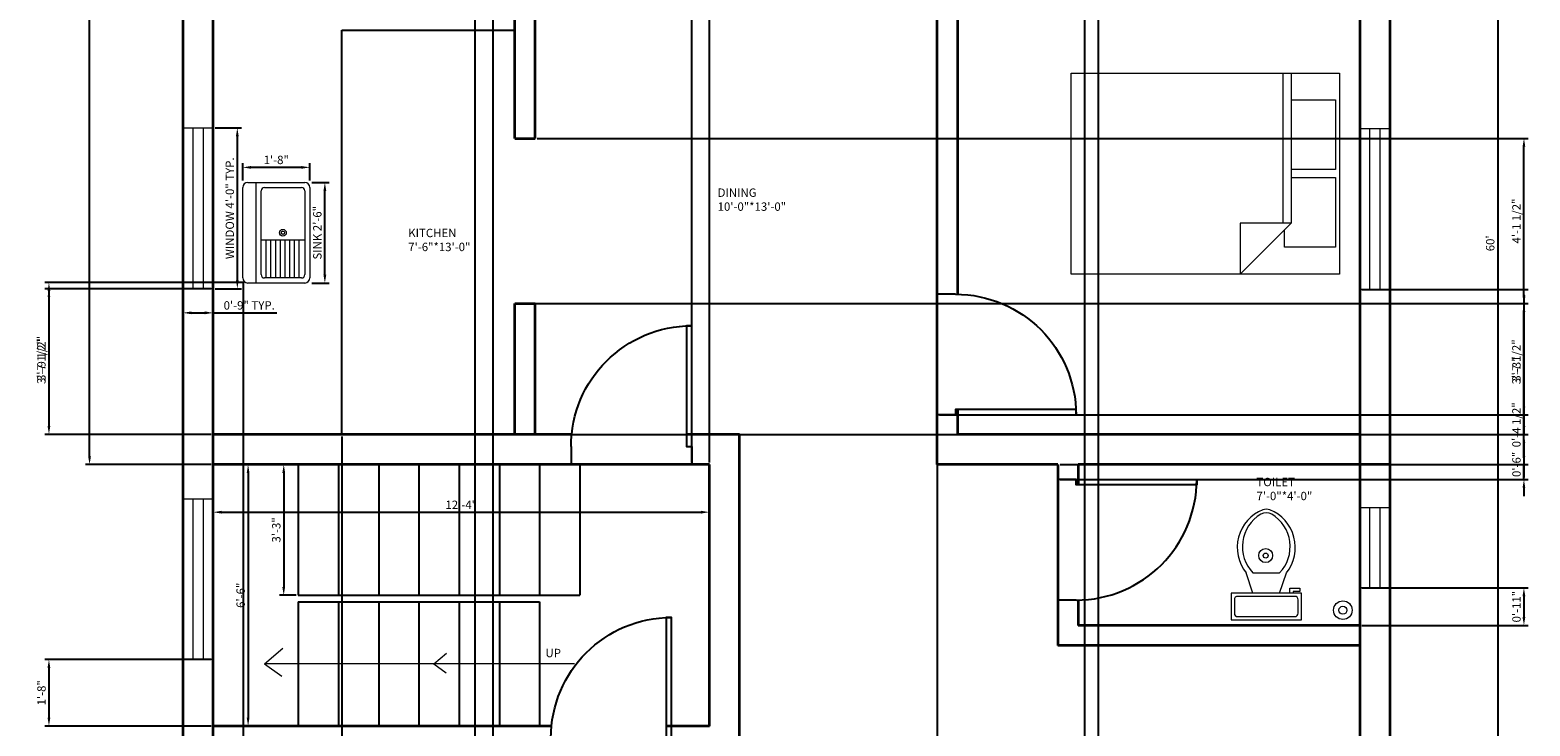
# Model space of a CAD drawing. Units: inches. Extents: x 2162 to 2610, y 1546 to 2356.
# Tile 2 of 3: x 2162 to 2610, y 1804 to 2012. Entities that reach past the tile are written whole.
import ezdxf

# ---------------------------------------------------------------- set-up
doc = ezdxf.new("R2010")
doc.units = ezdxf.units.IN
for name, color, linetype, lineweight in [('A-ANNO-DIMS', 2, 'Continuous', 18), ('A-ANNO-SYMB', 7, 'Continuous', 18), ('A-ANNO-TEXT', 7, 'Continuous', 25), ('A-AREA-IDEN', 7, 'Continuous', 18), ('A-DOOR', 3, 'Continuous', 25), ('A-FLOR-CASE', 8, 'Continuous', 25), ('A-FLOR-FIXT', 9, 'Continuous', 18), ('A-FLOR-STRS', 7, 'Continuous', 25), ('A-FURN', 8, 'Continuous', 18), ('A-GLAZ', 4, 'Continuous', 18), ('A-WALL', 7, 'Continuous', 35)]:
    doc.layers.add(name, color=color, linetype=linetype, lineweight=lineweight)
doc.styles.get("Standard").update_dxf_attribs({"font": 'arial.ttf'})
doc.dimstyles.new('ISO-25', dxfattribs={"dimtxt": 2.5, "dimasz": 2.5, "dimexe": 1.25, "dimexo": 0.625, "dimtad": 1, "dimdec": 1, "dimlunit": 3, "dimtxsty": 'Standard', "dimcen": 2.5, "dimadec": 0, "dimazin": 0, "dimtfac": 1, "dimtdec": 1, "dimtmove": 0, "dimatfit": 3, "dimfxl": 1, "dimarcsym": 0})

# ---------------------------------------------------------------- blocks, each defined once
blk = doc.blocks.new('*U2')
for p, q in [((0, 0), (0, -6)), ((40, 0), (40, -6))]:
    blk.add_line(p, q)
blk.add_lwpolyline([(0, 0), (0, 40), (1.75, 40), (1.75, 0)], close=True)
blk.add_arc((0, 0), 40, 0, 90)
blk = doc.blocks.new('*D4')
at = {"layer": 'A-ANNO-DIMS', "color": 0, "lineweight": -2, "transparency": 16777216}
for p, q in [((2216.24, 2308.05), (2178.74, 2308.05)), ((2179.99, 1884.55), (2179.99, 2305.55)), ((2216.24, 1882.05), (2178.74, 1882.05))]:
    blk.add_line(p, q, dxfattribs=at)
at = {"layer": 'A-ANNO-DIMS', "color": 0, "transparency": 16777216}
for points in [[(2179.57, 2305.55), (2180.4, 2305.55), (2179.99, 2308.05)], [(2179.57, 1884.55), (2180.4, 1884.55), (2179.99, 1882.05)]]:
    blk.add_solid(points, dxfattribs=at)
at = {"layer": 'Defpoints', "color": 0, "transparency": 16777216}
for p in [(2179.99, 2308.05), (2216.87, 2308.05), (2216.87, 1882.05)]:
    blk.add_point(p, dxfattribs=at)
at = {"layer": 'A-ANNO-DIMS', "color": 0, "transparency": 16777216, "insert": (2178.09, 2095.05), "char_height": 2.5, "attachment_point": 5, "rotation": 90}
blk.add_mtext('35\'-6"', dxfattribs=at)
blk = doc.blocks.new('*D5')
at = {"layer": 'A-ANNO-DIMS', "color": 0, "lineweight": -2, "transparency": 16777216}
for p, q in [((2568.49, 2308.05), (2601.29, 2308.05)), ((2600.04, 2305.55), (2600.04, 1590.55)), ((2568.49, 1588.05), (2601.29, 1588.05))]:
    blk.add_line(p, q, dxfattribs=at)
at = {"layer": 'A-ANNO-DIMS', "color": 0, "transparency": 16777216}
for points in [[(2599.62, 2305.55), (2600.45, 2305.55), (2600.04, 2308.05)], [(2599.62, 1590.55), (2600.45, 1590.55), (2600.04, 1588.05)]]:
    blk.add_solid(points, dxfattribs=at)
at = {"layer": 'Defpoints', "color": 0, "transparency": 16777216}
for p in [(2567.87, 2308.05), (2567.87, 1588.05), (2600.04, 1588.05)]:
    blk.add_point(p, dxfattribs=at)
at = {"layer": 'A-ANNO-DIMS', "color": 0, "transparency": 16777216, "insert": (2598.14, 1948.05), "char_height": 2.5, "attachment_point": 5, "rotation": 90}
blk.add_mtext("60'", dxfattribs=at)
blk = doc.blocks.new('Bed - Queen')
for p, q in [((0, -80.00003), (0, 0)), ((0, 0), (59.99999, 0)), ((59.99999, 0), (59.99999, -80.00003)), ((7.99999, -1.2), (28.79998, -1.2)), ((7.99999, -14.4), (7.99999, -1.2)), ((28.79998, -1.2), (28.79998, -14.4)), ((31.19999, -1.2), (51.99999, -1.2)), ((31.19999, -14.4), (31.19999, -1.2)), ((51.99999, -1.2), (51.99999, -16.4)), ((0, -14.4), (44.8, -14.4)), ((44.8, -16.8), (0, -16.8)), ((59.99999, -29.6), (44.8, -14.4)), ((44.8, -14.4), (44.8, -29.6)), ((51.99999, -16.4), (46.79936, -16.4)), ((44.8, -29.6), (59.99999, -29.6)), ((59.99999, -80.00003), (0, -80.00003))]:
    blk.add_line(p, q)
blk = doc.blocks.new('Toilet - top')
for p, q in [((9.5, -6), (9.5, -2)), ((-10, -8.5), (-8, -8.5)), ((-10, -9.5), (-10, -8.5)), ((-8, -8.5), (-8, -8)), ((-7, -8), (-7, -9.5)), ((-4, -8), (-6, -14)), ((4, -8), (6, -14)), ((-7, -9.5), (-10, -9.5)), ((4, -14), (-4, -14))]:
    blk.add_line(p, q)
blk.add_lwpolyline([(10.5, -8), (10.5, 0), (-10.5, 0), (-10.5, -8)], close=True)
for points in [[(-9.5, -2), (-9.5, -6)], [(8.5, -1), (-8.5, -1)], [(-8.5, -7), (8.5, -7)]]:
    blk.add_lwpolyline(points)
for centre, radius, start, end in [((-8.62, -1.88), 0.884, 81.8699, 188.1301), ((8.62, -1.88), 0.884, 351.8699, 98.1301), ((-8.62, -6.12), 0.884, 171.8699, 278.1301), ((8.62, -6.12), 0.884, 261.8699, 8.1301), ((3.52, -21.58), 12.17, 141.4691, 247.9714), ((4.2, -21.82), 11.33, 136.3677, 238.9468), ((-3.52, -21.58), 12.17, 292.0284, 38.5307), ((-4.2, -21.82), 11.33, 301.053, 43.6321), ((0, -27.88), 4, 245.7318, 294.2682), ((0, -29), 4, 254.8605, 285.1395)]:
    blk.add_arc(centre, radius, start, end)
blk = doc.blocks.new('Sink-single - 30 in top')
blk.add_line((-15, -3.999996), (15, -3.999996))
for points in [[(-13.5, 0), (13.5, 0)], [(-15, -18.499996), (-15, -1.5)], [(15, -1.5), (15, -18.499996)], [(-13.5, -17.499996), (-13.5, -6.499996)], [(-12.5, -5.499996), (12.5, -5.499996)], [(13.5, -6.499996), (13.5, -17.499996)], [(13.5, -19.999996), (-13.5, -19.999996)], [(12.5, -18.499996), (-12.5, -18.499996)]]:
    blk.add_lwpolyline(points)
for radius in [1, 0.5]:
    blk.add_circle((0, -11.999996), radius)
for centre, radius, start, end in [((-13.5, -1.5), 1.5, 90, 180), ((13.5, -1.5), 1.5, 0, 90), ((-12.5, -6.499996), 1, 90, 180), ((12.5, -6.499996), 1, 0, 90), ((-12.5, -17.499996), 1, 180, 270), ((12.5, -17.499996), 1, 270, 0), ((-13.5, -18.499996), 1.5, 180, 270), ((13.5, -18.499996), 1.5, 270, 0)]:
    blk.add_arc(centre, radius, start, end)
blk = doc.blocks.new('*D9')
at = {"layer": 'A-ANNO-DIMS', "color": 0, "lineweight": -2, "transparency": 16777216}
for p, q in [((2226.7, 1882.05), (2228.53, 1882.05)), ((2227.28, 1879.55), (2227.28, 1806.55)), ((2226.7, 1804.05), (2228.53, 1804.05))]:
    blk.add_line(p, q, dxfattribs=at)
at = {"layer": 'A-ANNO-DIMS', "color": 0, "transparency": 16777216}
for points in [[(2226.87, 1879.55), (2227.7, 1879.55), (2227.28, 1882.05)], [(2226.87, 1806.55), (2227.7, 1806.55), (2227.28, 1804.05)]]:
    blk.add_solid(points, dxfattribs=at)
at = {"layer": 'Defpoints', "color": 0, "transparency": 16777216}
for p in [(2226.07, 1882.05), (2226.07, 1804.05), (2227.28, 1804.05)]:
    blk.add_point(p, dxfattribs=at)
at = {"layer": 'A-ANNO-DIMS', "color": 0, "transparency": 16777216, "insert": (2225.38, 1843.05), "char_height": 2.5, "attachment_point": 5, "rotation": 90}
blk.add_mtext('6\'-6"', dxfattribs=at)
blk = doc.blocks.new('*D10')
at = {"layer": 'A-ANNO-DIMS', "color": 0, "lineweight": -2, "transparency": 16777216}
for p, q in [((2241.6, 1882.05), (2236.66, 1882.05)), ((2237.91, 1879.55), (2237.91, 1845.55)), ((2241.6, 1843.05), (2236.66, 1843.05))]:
    blk.add_line(p, q, dxfattribs=at)
at = {"layer": 'A-ANNO-DIMS', "color": 0, "transparency": 16777216}
for points in [[(2237.49, 1879.55), (2238.33, 1879.55), (2237.91, 1882.05)], [(2237.49, 1845.55), (2238.33, 1845.55), (2237.91, 1843.05)]]:
    blk.add_solid(points, dxfattribs=at)
at = {"layer": 'Defpoints', "color": 0, "transparency": 16777216}
for p in [(2242.23, 1882.05), (2237.91, 1843.05), (2242.23, 1843.05)]:
    blk.add_point(p, dxfattribs=at)
at = {"layer": 'A-ANNO-DIMS', "color": 0, "transparency": 16777216, "insert": (2236.01, 1862.55), "char_height": 2.5, "attachment_point": 5, "rotation": 90}
blk.add_mtext('3\'-3"', dxfattribs=at)
blk = doc.blocks.new('*D11')
at = {"layer": 'A-ANNO-DIMS', "color": 0, "lineweight": -2, "transparency": 16777216}
for p, q in [((2216.87, 1881.43), (2216.87, 1866.59)), ((2364.87, 1881.43), (2364.87, 1866.59)), ((2219.37, 1867.84), (2362.37, 1867.84))]:
    blk.add_line(p, q, dxfattribs=at)
at = {"layer": 'A-ANNO-DIMS', "color": 0, "transparency": 16777216}
for points in [[(2219.37, 1868.26), (2219.37, 1867.42), (2216.87, 1867.84)], [(2362.37, 1868.26), (2362.37, 1867.42), (2364.87, 1867.84)]]:
    blk.add_solid(points, dxfattribs=at)
at = {"layer": 'Defpoints', "color": 0, "transparency": 16777216}
for p in [(2216.87, 1882.05), (2364.87, 1882.05), (2364.87, 1867.84)]:
    blk.add_point(p, dxfattribs=at)
at = {"layer": 'A-ANNO-DIMS', "color": 0, "transparency": 16777216, "insert": (2290.87, 1869.72), "char_height": 2.5, "attachment_point": 5}
blk.add_mtext('12\'-4"', dxfattribs=at)
blk = doc.blocks.new('WIN-48IN')
for p, q in [((0, 0), (0, 48)), ((0, 48), (9, 48)), ((3, 0), (3, 48)), ((6, 48), (6, 0)), ((9, 48), (9, 0)), ((9, 0), (0, 0))]:
    blk.add_line(p, q)
blk = doc.blocks.new('WIN-24IN')
for p, q in [((0, 9), (24, 9)), ((0, 0), (0, 9)), ((24, 9), (24, 0)), ((0, 6), (24, 6)), ((24, 3), (0, 3)), ((24, 0), (0, 0))]:
    blk.add_line(p, q)
blk = doc.blocks.new('*D14')
at = {"layer": 'A-ANNO-DIMS', "color": 0, "lineweight": -2, "transparency": 16777216}
for p, q in [((2217.49, 1982.51), (2225.32, 1982.51)), ((2224.07, 1937.01), (2224.07, 1980.01)), ((2217.49, 1934.51), (2225.32, 1934.51))]:
    blk.add_line(p, q, dxfattribs=at)
at = {"layer": 'A-ANNO-DIMS', "color": 0, "transparency": 16777216}
for points in [[(2223.65, 1980.01), (2224.48, 1980.01), (2224.07, 1982.51)], [(2223.65, 1937.01), (2224.48, 1937.01), (2224.07, 1934.51)]]:
    blk.add_solid(points, dxfattribs=at)
at = {"layer": 'Defpoints', "color": 0, "transparency": 16777216}
for p in [(2216.87, 1982.51), (2224.07, 1982.51), (2216.87, 1934.51)]:
    blk.add_point(p, dxfattribs=at)
at = {"layer": 'A-ANNO-DIMS', "color": 0, "transparency": 16777216, "insert": (2222.15, 1958.51), "char_height": 2.5, "attachment_point": 5, "rotation": 90}
blk.add_mtext('WINDOW 4\'-0" TYP.', dxfattribs=at)
blk = doc.blocks.new('*D15')
at = {"layer": 'A-ANNO-DIMS', "color": 0, "lineweight": -2, "transparency": 16777216}
for p, q in [((2207.87, 1933.89), (2207.87, 1926.06)), ((2216.87, 1933.89), (2216.87, 1926.06)), ((2210.37, 1927.31), (2214.37, 1927.31)), ((2216.87, 1927.31), (2235.86, 1927.31))]:
    blk.add_line(p, q, dxfattribs=at)
at = {"layer": 'A-ANNO-DIMS', "color": 0, "transparency": 16777216}
for points in [[(2210.37, 1927.73), (2210.37, 1926.89), (2207.87, 1927.31)], [(2214.37, 1927.73), (2214.37, 1926.89), (2216.87, 1927.31)]]:
    blk.add_solid(points, dxfattribs=at)
at = {"layer": 'Defpoints', "color": 0, "transparency": 16777216}
for p in [(2207.87, 1934.51), (2216.87, 1934.51), (2216.87, 1927.31)]:
    blk.add_point(p, dxfattribs=at)
at = {"layer": 'A-ANNO-DIMS', "color": 0, "transparency": 16777216, "insert": (2227.61, 1929.21), "char_height": 2.5, "attachment_point": 5}
blk.add_mtext('0\'-9" TYP.', dxfattribs=at)
blk = doc.blocks.new('*D22')
at = {"layer": 'A-ANNO-DIMS', "color": 0, "lineweight": -2, "transparency": 16777216}
for p, q in [((2246.3, 1966.21), (2251.43, 1966.21)), ((2250.18, 1938.71), (2250.18, 1963.71)), ((2246.3, 1936.21), (2251.43, 1936.21))]:
    blk.add_line(p, q, dxfattribs=at)
at = {"layer": 'A-ANNO-DIMS', "color": 0, "transparency": 16777216}
for points in [[(2249.76, 1963.71), (2250.6, 1963.71), (2250.18, 1966.21)], [(2249.76, 1938.71), (2250.6, 1938.71), (2250.18, 1936.21)]]:
    blk.add_solid(points, dxfattribs=at)
at = {"layer": 'Defpoints', "color": 0, "transparency": 16777216}
for p in [(2245.68, 1966.21), (2250.18, 1966.21), (2245.68, 1936.21)]:
    blk.add_point(p, dxfattribs=at)
at = {"layer": 'A-ANNO-DIMS', "color": 0, "transparency": 16777216, "insert": (2248.26, 1951.21), "char_height": 2.5, "attachment_point": 5, "rotation": 90}
blk.add_mtext('SINK 2\'-6"', dxfattribs=at)
blk = doc.blocks.new('*D23')
at = {"layer": 'A-ANNO-DIMS', "color": 0, "lineweight": -2, "transparency": 16777216}
for p, q in [((2225.68, 1966.83), (2225.68, 1971.96)), ((2243.18, 1970.71), (2228.18, 1970.71)), ((2245.68, 1966.83), (2245.68, 1971.96))]:
    blk.add_line(p, q, dxfattribs=at)
at = {"layer": 'A-ANNO-DIMS', "color": 0, "transparency": 16777216}
for points in [[(2228.18, 1971.12), (2228.18, 1970.29), (2225.68, 1970.71)], [(2243.18, 1971.12), (2243.18, 1970.29), (2245.68, 1970.71)]]:
    blk.add_solid(points, dxfattribs=at)
at = {"layer": 'Defpoints', "color": 0, "transparency": 16777216}
for p in [(2225.68, 1970.71), (2225.68, 1966.21), (2245.68, 1966.21)]:
    blk.add_point(p, dxfattribs=at)
at = {"layer": 'A-ANNO-DIMS', "color": 0, "transparency": 16777216, "insert": (2235.68, 1972.61), "char_height": 2.5, "attachment_point": 5}
blk.add_mtext('1\'-8"', dxfattribs=at)
blk = doc.blocks.new('*D25')
at = {"layer": 'A-ANNO-DIMS', "color": 0, "lineweight": -2, "transparency": 16777216}
for p, q in [((2313.49, 1979.36), (2609.12, 1979.36)), ((2607.87, 1932.55), (2607.87, 1976.86)), ((2313.49, 1930.05), (2609.12, 1930.05))]:
    blk.add_line(p, q, dxfattribs=at)
at = {"layer": 'A-ANNO-DIMS', "color": 0, "transparency": 16777216}
for points in [[(2607.45, 1976.86), (2608.28, 1976.86), (2607.87, 1979.36)], [(2607.45, 1932.55), (2608.28, 1932.55), (2607.87, 1930.05)]]:
    blk.add_solid(points, dxfattribs=at)
at = {"layer": 'Defpoints', "color": 0, "transparency": 16777216}
for p in [(2312.87, 1979.36), (2607.87, 1979.36), (2312.87, 1930.05)]:
    blk.add_point(p, dxfattribs=at)
at = {"layer": 'A-ANNO-DIMS', "color": 0, "transparency": 16777216, "insert": (2605.95, 1954.71), "char_height": 2.5, "attachment_point": 5, "rotation": 90}
blk.add_mtext('4\'-1 1/2"', dxfattribs=at)
blk = doc.blocks.new('*D26')
at = {"layer": 'A-ANNO-DIMS', "color": 0, "lineweight": -2, "transparency": 16777216}
for p, q in [((2432.87, 1896.22), (2432.87, 1546.8)), ((2373.87, 1890.43), (2373.87, 1546.8)), ((2376.37, 1548.05), (2430.37, 1548.05))]:
    blk.add_line(p, q, dxfattribs=at)
at = {"layer": 'A-ANNO-DIMS', "color": 0, "transparency": 16777216}
for points in [[(2376.37, 1548.47), (2376.37, 1547.63), (2373.87, 1548.05)], [(2430.37, 1548.47), (2430.37, 1547.63), (2432.87, 1548.05)]]:
    blk.add_solid(points, dxfattribs=at)
at = {"layer": 'Defpoints', "color": 0, "transparency": 16777216}
for p in [(2432.87, 1896.85), (2373.87, 1891.05), (2432.87, 1548.05)]:
    blk.add_point(p, dxfattribs=at)
at = {"layer": 'A-ANNO-DIMS', "color": 0, "transparency": 16777216, "insert": (2403.37, 1549.93), "char_height": 2.5, "attachment_point": 5}
blk.add_mtext('4\'-11"', dxfattribs=at)
blk = doc.blocks.new('*D28')
at = {"layer": 'A-ANNO-DIMS', "color": 0, "lineweight": -2, "transparency": 16777216}
for p, q in [((2216.24, 1934.51), (2166.62, 1934.51)), ((2167.87, 1932.01), (2167.87, 1893.55)), ((2216.24, 1891.05), (2166.62, 1891.05))]:
    blk.add_line(p, q, dxfattribs=at)
at = {"layer": 'A-ANNO-DIMS', "color": 0, "transparency": 16777216}
for points in [[(2167.45, 1932.01), (2168.28, 1932.01), (2167.87, 1934.51)], [(2167.45, 1893.55), (2168.28, 1893.55), (2167.87, 1891.05)]]:
    blk.add_solid(points, dxfattribs=at)
at = {"layer": 'Defpoints', "color": 0, "transparency": 16777216}
for p in [(2216.87, 1934.51), (2167.87, 1891.05), (2216.87, 1891.05)]:
    blk.add_point(p, dxfattribs=at)
at = {"layer": 'A-ANNO-DIMS', "color": 0, "transparency": 16777216, "insert": (2165.95, 1912.78), "char_height": 2.5, "attachment_point": 5, "rotation": 90}
blk.add_mtext('3\'-7 1/2"', dxfattribs=at)
blk = doc.blocks.new('*D29')
at = {"layer": 'A-ANNO-DIMS', "color": 0, "lineweight": -2, "transparency": 16777216}
for p, q in [((2216.24, 1823.87), (2166.62, 1823.87)), ((2167.87, 1821.37), (2167.87, 1806.55)), ((2216.24, 1804.05), (2166.62, 1804.05))]:
    blk.add_line(p, q, dxfattribs=at)
at = {"layer": 'A-ANNO-DIMS', "color": 0, "transparency": 16777216}
for points in [[(2167.45, 1821.37), (2168.28, 1821.37), (2167.87, 1823.87)], [(2167.45, 1806.55), (2168.28, 1806.55), (2167.87, 1804.05)]]:
    blk.add_solid(points, dxfattribs=at)
at = {"layer": 'Defpoints', "color": 0, "transparency": 16777216}
for p in [(2216.87, 1823.87), (2167.87, 1804.05), (2216.87, 1804.05)]:
    blk.add_point(p, dxfattribs=at)
at = {"layer": 'A-ANNO-DIMS', "color": 0, "transparency": 16777216, "insert": (2165.97, 1813.96), "char_height": 2.5, "attachment_point": 5, "rotation": 90}
blk.add_mtext('1\'-8"', dxfattribs=at)
blk = doc.blocks.new('*D31')
at = {"layer": 'A-ANNO-DIMS', "color": 0, "lineweight": -2, "transparency": 16777216}
for p, q in [((2559.49, 1934.32), (2609.12, 1934.32)), ((2607.87, 1931.82), (2607.87, 1893.55)), ((2559.49, 1891.05), (2609.12, 1891.05))]:
    blk.add_line(p, q, dxfattribs=at)
at = {"layer": 'A-ANNO-DIMS', "color": 0, "transparency": 16777216}
for points in [[(2607.45, 1931.82), (2608.28, 1931.82), (2607.87, 1934.32)], [(2607.45, 1893.55), (2608.28, 1893.55), (2607.87, 1891.05)]]:
    blk.add_solid(points, dxfattribs=at)
at = {"layer": 'Defpoints', "color": 0, "transparency": 16777216}
for p in [(2558.87, 1934.32), (2558.87, 1891.05), (2607.87, 1891.05)]:
    blk.add_point(p, dxfattribs=at)
at = {"layer": 'A-ANNO-DIMS', "color": 0, "transparency": 16777216, "insert": (2605.95, 1912.69), "char_height": 2.5, "attachment_point": 5, "rotation": 90}
blk.add_mtext('3\'-7 1/2"', dxfattribs=at)
blk = doc.blocks.new('*D32')
at = {"layer": 'A-ANNO-DIMS', "color": 0, "lineweight": -2, "transparency": 16777216}
for p, q in [((2559.49, 1845.27), (2609.12, 1845.27)), ((2607.87, 1842.77), (2607.87, 1836.55)), ((2559.49, 1834.05), (2609.12, 1834.05))]:
    blk.add_line(p, q, dxfattribs=at)
at = {"layer": 'A-ANNO-DIMS', "color": 0, "transparency": 16777216}
for points in [[(2607.45, 1842.77), (2608.28, 1842.77), (2607.87, 1845.27)], [(2607.45, 1836.55), (2608.28, 1836.55), (2607.87, 1834.05)]]:
    blk.add_solid(points, dxfattribs=at)
at = {"layer": 'Defpoints', "color": 0, "transparency": 16777216}
for p in [(2558.87, 1845.27), (2558.87, 1834.05), (2607.87, 1834.05)]:
    blk.add_point(p, dxfattribs=at)
at = {"layer": 'A-ANNO-DIMS', "color": 0, "transparency": 16777216, "insert": (2605.97, 1839.66), "char_height": 2.5, "attachment_point": 5, "rotation": 90}
blk.add_mtext('0\'-11"', dxfattribs=at)
blk = doc.blocks.new('*D40')
at = {"layer": 'A-ANNO-DIMS', "color": 0, "lineweight": -2, "transparency": 16777216}
for p, q in [((2216.87, 1890.43), (2216.87, 1546.8)), ((2255.27, 1890.43), (2255.27, 1546.8)), ((2219.37, 1548.05), (2252.77, 1548.05))]:
    blk.add_line(p, q, dxfattribs=at)
at = {"layer": 'A-ANNO-DIMS', "color": 0, "transparency": 16777216}
for points in [[(2219.37, 1548.47), (2219.37, 1547.63), (2216.87, 1548.05)], [(2252.77, 1548.47), (2252.77, 1547.63), (2255.27, 1548.05)]]:
    blk.add_solid(points, dxfattribs=at)
at = {"layer": 'Defpoints', "color": 0, "transparency": 16777216}
for p in [(2216.87, 1891.05), (2255.27, 1891.05), (2255.27, 1548.05)]:
    blk.add_point(p, dxfattribs=at)
at = {"layer": 'A-ANNO-DIMS', "color": 0, "transparency": 16777216, "insert": (2236.07, 1549.97), "char_height": 2.5, "attachment_point": 5}
blk.add_mtext('3\'-2 1/2"', dxfattribs=at)
blk = doc.blocks.new('*D44')
at = {"layer": 'A-ANNO-DIMS', "color": 0, "lineweight": -2, "transparency": 16777216}
for p, q in [((2307.49, 1930.05), (2609.12, 1930.05)), ((2607.87, 1893.55), (2607.87, 1927.55)), ((2307.49, 1891.05), (2609.12, 1891.05))]:
    blk.add_line(p, q, dxfattribs=at)
at = {"layer": 'A-ANNO-DIMS', "color": 0, "transparency": 16777216}
for points in [[(2607.45, 1927.55), (2608.28, 1927.55), (2607.87, 1930.05)], [(2607.45, 1893.55), (2608.28, 1893.55), (2607.87, 1891.05)]]:
    blk.add_solid(points, dxfattribs=at)
at = {"layer": 'Defpoints', "color": 0, "transparency": 16777216}
for p in [(2306.87, 1930.05), (2607.87, 1930.05), (2306.87, 1891.05)]:
    blk.add_point(p, dxfattribs=at)
at = {"layer": 'A-ANNO-DIMS', "color": 0, "transparency": 16777216, "insert": (2605.96, 1910.55), "char_height": 2.5, "attachment_point": 5, "rotation": 90}
blk.add_mtext('3\'-3"', dxfattribs=at)
blk = doc.blocks.new('*D47')
at = {"layer": 'A-ANNO-DIMS', "color": 0, "lineweight": -2, "transparency": 16777216}
for p, q in [((2225.97, 1936.32), (2166.62, 1936.32)), ((2167.87, 1933.82), (2167.87, 1893.55)), ((2216.24, 1891.05), (2166.62, 1891.05))]:
    blk.add_line(p, q, dxfattribs=at)
at = {"layer": 'A-ANNO-DIMS', "color": 0, "transparency": 16777216}
for points in [[(2167.45, 1933.82), (2168.28, 1933.82), (2167.87, 1936.32)], [(2167.45, 1893.55), (2168.28, 1893.55), (2167.87, 1891.05)]]:
    blk.add_solid(points, dxfattribs=at)
at = {"layer": 'Defpoints', "color": 0, "transparency": 16777216}
for p in [(2226.6, 1936.32), (2167.87, 1891.05), (2216.87, 1891.05)]:
    blk.add_point(p, dxfattribs=at)
at = {"layer": 'A-ANNO-DIMS', "color": 0, "transparency": 16777216, "insert": (2165.95, 1913.69), "char_height": 2.5, "attachment_point": 5, "rotation": 90}
blk.add_mtext('3\'-9 1/2"', dxfattribs=at)
blk = doc.blocks.new('*D48')
at = {"layer": 'A-ANNO-DIMS', "color": 0, "lineweight": -2, "transparency": 16777216}
for p, q in [((2216.87, 1933.89), (2216.87, 1546.8)), ((2225.8, 1936.5), (2225.8, 1546.8)), ((2223.3, 1548.05), (2219.37, 1548.05))]:
    blk.add_line(p, q, dxfattribs=at)
at = {"layer": 'A-ANNO-DIMS', "color": 0, "transparency": 16777216}
for points in [[(2219.37, 1548.47), (2219.37, 1547.63), (2216.87, 1548.05)], [(2223.3, 1548.47), (2223.3, 1547.63), (2225.8, 1548.05)]]:
    blk.add_solid(points, dxfattribs=at)
at = {"layer": 'Defpoints', "color": 0, "transparency": 16777216}
for p in [(2216.87, 1934.51), (2225.8, 1937.12), (2216.87, 1548.05)]:
    blk.add_point(p, dxfattribs=at)
at = {"layer": 'A-ANNO-DIMS', "color": 0, "transparency": 16777216, "insert": (2221.33, 1549.95), "char_height": 2.5, "attachment_point": 5}
blk.add_mtext('0\'-9"', dxfattribs=at)
blk = doc.blocks.new('*D50')
at = {"layer": 'A-ANNO-DIMS', "color": 0, "lineweight": -2, "transparency": 16777216}
for p, q in [((2359.63, 1882.68), (2359.63, 2349.3)), ((2364.87, 1882.68), (2364.87, 2349.3)), ((2357.13, 2348.05), (2354.63, 2348.05)), ((2359.63, 2348.05), (2364.87, 2348.05)), ((2367.37, 2348.05), (2377.76, 2348.05))]:
    blk.add_line(p, q, dxfattribs=at)
at = {"layer": 'A-ANNO-DIMS', "color": 0, "transparency": 16777216}
for points in [[(2357.13, 2348.47), (2357.13, 2347.63), (2359.63, 2348.05)], [(2367.37, 2348.47), (2367.37, 2347.63), (2364.87, 2348.05)]]:
    blk.add_solid(points, dxfattribs=at)
at = {"layer": 'Defpoints', "color": 0, "transparency": 16777216}
for p in [(2364.87, 2348.05), (2359.63, 1882.05), (2364.87, 1882.05)]:
    blk.add_point(p, dxfattribs=at)
at = {"layer": 'A-ANNO-DIMS', "color": 0, "transparency": 16777216, "insert": (2373.81, 2349.95), "char_height": 2.5, "attachment_point": 5}
blk.add_mtext('0\'-5"', dxfattribs=at)
blk = doc.blocks.new('*D56')
at = {"layer": 'A-ANNO-DIMS', "color": 0, "lineweight": -2, "transparency": 16777216}
for p, q in [((2294.87, 2214.43), (2294.87, 1546.8)), ((2300.28, 2208.43), (2300.28, 1546.8)), ((2292.37, 1548.05), (2289.87, 1548.05)), ((2294.87, 1548.05), (2300.28, 1548.05)), ((2302.78, 1548.05), (2319.01, 1548.05))]:
    blk.add_line(p, q, dxfattribs=at)
at = {"layer": 'A-ANNO-DIMS', "color": 0, "transparency": 16777216}
for points in [[(2292.37, 1548.47), (2292.37, 1547.63), (2294.87, 1548.05)], [(2302.78, 1548.47), (2302.78, 1547.63), (2300.28, 1548.05)]]:
    blk.add_solid(points, dxfattribs=at)
at = {"layer": 'Defpoints', "color": 0, "transparency": 16777216}
for p in [(2294.87, 2215.05), (2300.28, 2209.05), (2300.28, 1548.05)]:
    blk.add_point(p, dxfattribs=at)
at = {"layer": 'A-ANNO-DIMS', "color": 0, "transparency": 16777216, "insert": (2312.14, 1549.97), "char_height": 2.5, "attachment_point": 5}
blk.add_mtext('0\'-5 1/2"', dxfattribs=at)
blk = doc.blocks.new('*D57')
at = {"layer": 'A-ANNO-DIMS', "color": 0, "lineweight": -2, "transparency": 16777216}
for p, q in [((2480.87, 2214.43), (2480.87, 1546.8)), ((2476.76, 2208.43), (2476.76, 1546.8)), ((2474.26, 1548.05), (2471.76, 1548.05)), ((2476.76, 1548.05), (2480.87, 1548.05)), ((2483.37, 1548.05), (2493.76, 1548.05))]:
    blk.add_line(p, q, dxfattribs=at)
at = {"layer": 'A-ANNO-DIMS', "color": 0, "transparency": 16777216}
for points in [[(2474.26, 1548.47), (2474.26, 1547.63), (2476.76, 1548.05)], [(2483.37, 1548.47), (2483.37, 1547.63), (2480.87, 1548.05)]]:
    blk.add_solid(points, dxfattribs=at)
at = {"layer": 'Defpoints', "color": 0, "transparency": 16777216}
for p in [(2480.87, 2215.05), (2476.76, 2209.05), (2480.87, 1548.05)]:
    blk.add_point(p, dxfattribs=at)
at = {"layer": 'A-ANNO-DIMS', "color": 0, "transparency": 16777216, "insert": (2489.81, 1549.95), "char_height": 2.5, "attachment_point": 5}
blk.add_mtext('0\'-4"', dxfattribs=at)
blk = doc.blocks.new('*D59')
at = {"layer": 'A-ANNO-DIMS', "color": 0, "lineweight": -2, "transparency": 16777216}
for p, q in [((2607.87, 1899.35), (2607.87, 1901.85)), ((2433.49, 1896.85), (2609.12, 1896.85)), ((2607.87, 1896.85), (2607.87, 1891.05)), ((2439.49, 1891.05), (2609.12, 1891.05)), ((2607.87, 1888.55), (2607.87, 1878.16))]:
    blk.add_line(p, q, dxfattribs=at)
at = {"layer": 'A-ANNO-DIMS', "color": 0, "transparency": 16777216}
for points in [[(2607.45, 1899.35), (2608.28, 1899.35), (2607.87, 1896.85)], [(2607.45, 1888.55), (2608.28, 1888.55), (2607.87, 1891.05)]]:
    blk.add_solid(points, dxfattribs=at)
at = {"layer": 'Defpoints', "color": 0, "transparency": 16777216}
for p in [(2432.87, 1896.85), (2438.87, 1891.05), (2607.87, 1891.05)]:
    blk.add_point(p, dxfattribs=at)
at = {"layer": 'A-ANNO-DIMS', "color": 0, "transparency": 16777216, "insert": (2605.97, 1882.1), "char_height": 2.5, "attachment_point": 5, "rotation": 90}
blk.add_mtext('0\'-6"', dxfattribs=at)
blk = doc.blocks.new('*D60')
at = {"layer": 'A-ANNO-DIMS', "color": 0, "lineweight": -2, "transparency": 16777216}
for p, q in [((2607.87, 1884.55), (2607.87, 1900.77)), ((2469.49, 1882.05), (2609.12, 1882.05)), ((2607.87, 1877.61), (2607.87, 1882.05)), ((2469.49, 1877.61), (2609.12, 1877.61)), ((2607.87, 1875.11), (2607.87, 1872.61))]:
    blk.add_line(p, q, dxfattribs=at)
at = {"layer": 'A-ANNO-DIMS', "color": 0, "transparency": 16777216}
for points in [[(2607.45, 1884.55), (2608.28, 1884.55), (2607.87, 1882.05)], [(2607.45, 1875.11), (2608.28, 1875.11), (2607.87, 1877.61)]]:
    blk.add_solid(points, dxfattribs=at)
at = {"layer": 'Defpoints', "color": 0, "transparency": 16777216}
for p in [(2468.87, 1882.05), (2607.87, 1882.05), (2468.87, 1877.61)]:
    blk.add_point(p, dxfattribs=at)
at = {"layer": 'A-ANNO-DIMS', "color": 0, "transparency": 16777216, "insert": (2605.95, 1893.91), "char_height": 2.5, "attachment_point": 5, "rotation": 90}
blk.add_mtext('0\'-4 1/2"', dxfattribs=at)

msp = doc.modelspace()

# ---------------------------------------------------------------- linework, layer by layer
at = {"layer": 'A-ANNO-SYMB'}
for p, q in [((2232.18, 1822.55), (2237.69, 1827.28)), ((2282.67, 1822.55), (2286.45, 1825.8)), ((2324.65, 1822.55), (2232.18, 1822.55)), ((2232.18, 1822.55), (2237.36, 1818.88)), ((2282.67, 1822.55), (2286.38, 1819.89))]:
    msp.add_line(p, q, dxfattribs=at)
at = {"layer": 'A-FLOR-CASE'}
for p, q in [((2255.27, 1891.05), (2255.27, 2011.69)), ((2255.27, 2011.69), (2306.87, 2011.69))]:
    msp.add_line(p, q, dxfattribs=at)
at = {"layer": 'A-FLOR-FIXT'}
for p, q in [((2231.18, 1949.1), (2244.18, 1949.1)), ((2232.61, 1949.1), (2232.61, 1937.71)), ((2234.01, 1949.1), (2234.01, 1937.71)), ((2235.41, 1949.1), (2235.41, 1937.71)), ((2236.81, 1949.1), (2236.81, 1937.71)), ((2238.21, 1949.1), (2238.21, 1937.71)), ((2239.61, 1949.1), (2239.61, 1937.71)), ((2241.01, 1949.1), (2241.01, 1937.71)), ((2242.41, 1949.1), (2242.41, 1937.71))]:
    msp.add_line(p, q, dxfattribs=at)
for centre, radius in [((2530.83, 1854.89), 2.08), ((2530.83, 1854.89), 0.742), ((2553.86, 1838.6), 2.77), ((2553.86, 1838.6), 1.2)]:
    msp.add_circle(centre, radius, dxfattribs=at)
at = {"layer": 'A-FLOR-STRS'}
for p, q in [((2242.23, 1882.05), (2242.23, 1843.05)), ((2254.23, 1882.05), (2254.23, 1843.05)), ((2266.23, 1882.05), (2266.23, 1843.05)), ((2278.23, 1882.05), (2278.23, 1843.05)), ((2290.23, 1882.05), (2290.23, 1843.05)), ((2302.23, 1882.05), (2302.23, 1843.05)), ((2314.23, 1882.05), (2314.23, 1843.05)), ((2326.23, 1882.05), (2326.23, 1843.05)), ((2242.23, 1843.05), (2326.23, 1843.05)), ((2242.23, 1841.05), (2314.23, 1841.05)), ((2242.23, 1841.05), (2242.23, 1804.05)), ((2254.23, 1841.05), (2254.23, 1804.05)), ((2266.23, 1841.05), (2266.23, 1804.05)), ((2278.23, 1841.05), (2278.23, 1804.05)), ((2290.23, 1841.05), (2290.23, 1804.05)), ((2302.23, 1841.05), (2302.23, 1804.05)), ((2314.23, 1841.05), (2314.23, 1804.05))]:
    msp.add_line(p, q, dxfattribs=at)
at = {"layer": 'A-WALL'}
for p, q in [((2207.87, 1588.05), (2207.87, 2308.05)), ((2567.87, 2308.05), (2567.87, 1588.05)), ((2216.87, 1588.05), (2216.87, 2299.05)), ((2558.87, 2299.05), (2558.87, 1595.05)), ((2438.87, 2052.55), (2438.87, 1932.84)), ((2306.87, 1979.36), (2306.87, 2046.55)), ((2312.87, 1979.36), (2312.87, 2046.55)), ((2432.87, 1882.05), (2432.87, 2046.55)), ((2306.87, 1979.36), (2312.87, 1979.36)), ((2306.87, 1891.05), (2306.87, 1930.05)), ((2306.87, 1930.05), (2312.87, 1930.05)), ((2312.87, 1891.05), (2312.87, 1930.05)), ((2438.87, 1898.42), (2438.87, 1891.05)), ((2323.81, 1891.05), (2216.87, 1891.05)), ((2373.87, 1891.05), (2358.06, 1891.05)), ((2373.87, 1707.57), (2373.87, 1891.05)), ((2558.87, 1891.05), (2438.87, 1891.05)), ((2364.87, 1882.05), (2216.87, 1882.05)), ((2364.87, 1804.05), (2364.87, 1882.05)), ((2468.87, 1882.05), (2432.87, 1882.05)), ((2468.87, 1882.05), (2468.87, 1828.05)), ((2567.87, 1882.05), (2474.87, 1882.05)), ((2474.87, 1882.05), (2474.87, 1876.04)), ((2474.87, 1841.62), (2474.87, 1834.05)), ((2558.87, 1834.05), (2474.87, 1834.05)), ((2558.87, 1828.05), (2468.87, 1828.05)), ((2317.79, 1804.05), (2216.87, 1804.05)), ((2364.87, 1804.05), (2352.03, 1804.05))]:
    msp.add_line(p, q, dxfattribs=at)

# ---------------------------------------------------------------- block references
at = {"layer": 'A-DOOR', "yscale": 0.9, "zscale": 0.9, "rotation": 270}
for p, xscale in [((2438.27, 1896.85), -0.9), ((2474.27, 1877.61), 0.9)]:
    msp.add_blockref('*U2', p, dxfattribs=dict(at, xscale=xscale))
at = {"layer": 'A-DOOR', "xscale": -0.9, "yscale": 0.9, "zscale": 0.9}
for p in [(2359.63, 1887.45), (2353.61, 1800.45)]:
    msp.add_blockref('*U2', p, dxfattribs=at)
at = {"layer": 'A-FLOR-FIXT'}
for name, p, rotation in [('Sink-single - 30 in top', (2225.68, 1951.21), 90), ('Toilet - top', (2531, 1835.72), 180)]:
    msp.add_blockref(name, p, dxfattribs=dict(at, rotation=rotation))
at = {"layer": 'A-FURN', "rotation": 270}
msp.add_blockref('Bed - Queen', (2552.83, 1998.86), dxfattribs=at)
at = {"layer": 'A-GLAZ'}
for p in [(2207.87, 1934.51), (2558.87, 1934.32), (2207.87, 1823.87)]:
    msp.add_blockref('WIN-48IN', p, dxfattribs=at)
at = {"layer": 'A-GLAZ', "rotation": 90.0000000000012}
msp.add_blockref('WIN-24IN', (2567.87, 1845.27), dxfattribs=at)

# ---------------------------------------------------------------- texts
at = {"layer": 'A-ANNO-TEXT', "insert": (2315.98, 1827.08), "char_height": 2.5, "attachment_point": 1}
msp.add_mtext_dynamic_manual_height_columns('UP', width=7.1916, gutter_width=12.5, heights=[0], dxfattribs=at)
at = {"layer": 'A-AREA-IDEN', "char_height": 2.5, "attachment_point": 1}
for s, width, insert in [('DINING\\P10\'-0"*13\'-0"', 73.2252, (2367.34, 1964.42)), ('KITCHEN\\P7\'-6"*13\'-0"', 44.1055, (2275.06, 1952.39)), ('TOILET\\P7\'-0"*4\'-0"', 43.2123, (2528.08, 1878.09))]:
    msp.add_mtext_dynamic_manual_height_columns(s, width=width, gutter_width=12.5, heights=[0], dxfattribs=dict(at, insert=insert))

# ---------------------------------------------------------------- dimensions: what is measured, and where the dimension line sits
at = {"layer": 'A-ANNO-DIMS'}
for base, p1, p2, override, picture, middle in [((2364.87, 2348.05), (2359.63, 1882.05), (2364.87, 1882.05), {"dimdec": 1, "dimlfac": 1, "dimrnd": 0, "dimzin": 1, "dimdsep": 46, "dimlunit": 4, "dimfrac": 2}, '*D50', (2373.81, 2349.95)), ((2300.28, 1548.05), (2294.87, 2215.05), (2300.28, 2209.05), {"dimdec": 1, "dimlfac": 1, "dimrnd": 0, "dimzin": 1, "dimdsep": 46, "dimlunit": 4, "dimfrac": 2}, '*D56', (2312.14, 1549.97)), ((2480.87, 1548.05), (2476.76, 2209.05), (2480.87, 2215.05), {"dimdec": 1, "dimlfac": 1, "dimrnd": 0, "dimzin": 1, "dimdsep": 46, "dimlunit": 4, "dimfrac": 2}, '*D57', (2489.81, 1549.95)), ((2216.87, 1548.05), (2225.8, 1937.12), (2216.87, 1934.51), {"dimdec": 1, "dimlfac": 1, "dimrnd": 0, "dimzin": 1, "dimdsep": 46, "dimlunit": 4, "dimfrac": 2}, '*D48', (2221.33, 1549.95)), ((2432.87, 1548.05), (2373.87, 1891.05), (2432.87, 1896.85), {"dimdec": 1, "dimlfac": 1, "dimrnd": 0, "dimzin": 1, "dimdsep": 46, "dimlunit": 4, "dimfrac": 2}, '*D26', (2403.37, 1549.93)), ((2255.27, 1548.05), (2216.87, 1891.05), (2255.27, 1891.05), {"dimdec": 1, "dimlfac": 1, "dimrnd": 0, "dimzin": 1, "dimdsep": 46, "dimlunit": 4, "dimfrac": 2}, '*D40', (2236.07, 1549.97)), ((2364.87, 1867.84), (2216.87, 1882.05), (2364.87, 1882.05), {"dimclrd": 0, "dimclre": 0, "dimclrt": 0}, '*D11', (2290.87, 1869.72))]:
    dim = msp.add_linear_dim(base=base, p1=p1, p2=p2, dimstyle='ISO-25', override=override, dxfattribs=at)
    dim.commit()
    dim.dimension.update_dxf_attribs({"geometry": picture, "text_midpoint": middle})
for base, p1, p2, angle, override, picture, middle in [((2179.99, 2308.05), (2216.87, 1882.05), (2216.87, 2308.05), 90, {"dimclrd": 0, "dimclre": 0, "dimclrt": 0}, '*D4', (2178.09, 2095.05)), ((2600.04, 1588.05), (2567.87, 2308.05), (2567.87, 1588.05), 90, {"dimclrd": 0, "dimclre": 0, "dimclrt": 0}, '*D5', (2598.14, 1948.05)), ((2607.87, 1979.36), (2312.87, 1930.05), (2312.87, 1979.36), 90, {"dimdec": 1, "dimlfac": 1, "dimrnd": 0, "dimzin": 1, "dimdsep": 46, "dimlunit": 4, "dimfrac": 2}, '*D25', (2605.95, 1954.71)), ((2225.68, 1970.71), (2245.68, 1966.21), (2225.68, 1966.21), 180, {"dimdec": 1, "dimlfac": 1, "dimrnd": 0, "dimzin": 1, "dimdsep": 46, "dimlunit": 4, "dimfrac": 2}, '*D23', (2235.68, 1972.61)), ((2167.87, 1891.05), (2226.6, 1936.32), (2216.87, 1891.05), 90, {"dimdec": 1, "dimlfac": 1, "dimrnd": 0, "dimzin": 1, "dimdsep": 46, "dimlunit": 4, "dimfrac": 2}, '*D47', (2165.95, 1913.69)), ((2167.87, 1891.05), (2216.87, 1934.51), (2216.87, 1891.05), 90, {"dimdec": 1, "dimlfac": 1, "dimrnd": 0, "dimzin": 1, "dimdsep": 46, "dimlunit": 4, "dimfrac": 2}, '*D28', (2165.95, 1912.78)), ((2607.87, 1891.05), (2558.87, 1934.32), (2558.87, 1891.05), 90, {"dimdec": 1, "dimlfac": 1, "dimrnd": 0, "dimzin": 1, "dimdsep": 46, "dimlunit": 4, "dimfrac": 2}, '*D31', (2605.95, 1912.69)), ((2607.87, 1930.05), (2306.87, 1891.05), (2306.87, 1930.05), 90, {"dimdec": 1, "dimlfac": 1, "dimrnd": 0, "dimzin": 1, "dimdsep": 46, "dimlunit": 4, "dimfrac": 2}, '*D44', (2605.96, 1910.55)), ((2607.87, 1891.05), (2432.87, 1896.85), (2438.87, 1891.05), 90, {"dimdec": 1, "dimlfac": 1, "dimrnd": 0, "dimzin": 1, "dimdsep": 46, "dimlunit": 4, "dimfrac": 2}, '*D59', (2605.97, 1882.1)), ((2607.87, 1882.05), (2468.87, 1877.61), (2468.87, 1882.05), 90, {"dimdec": 1, "dimlfac": 1, "dimrnd": 0, "dimzin": 1, "dimdsep": 46, "dimlunit": 4, "dimfrac": 2}, '*D60', (2605.95, 1893.91)), ((2227.28, 1804.05), (2226.07, 1882.05), (2226.07, 1804.05), 90, {"dimclrd": 0, "dimclre": 0, "dimclrt": 0}, '*D9', (2225.38, 1843.05)), ((2237.91, 1843.05), (2242.23, 1882.05), (2242.23, 1843.05), 90, {"dimclrd": 0, "dimclre": 0, "dimclrt": 0}, '*D10', (2236.01, 1862.55)), ((2607.87, 1834.05), (2558.87, 1845.27), (2558.87, 1834.05), 90, {"dimdec": 1, "dimlfac": 1, "dimrnd": 0, "dimzin": 1, "dimdsep": 46, "dimlunit": 4, "dimfrac": 2}, '*D32', (2605.97, 1839.66)), ((2167.87, 1804.05), (2216.87, 1823.87), (2216.87, 1804.05), 90, {"dimdec": 1, "dimlfac": 1, "dimrnd": 0, "dimzin": 1, "dimdsep": 46, "dimlunit": 4, "dimfrac": 2}, '*D29', (2165.97, 1813.96))]:
    dim = msp.add_linear_dim(base=base, p1=p1, p2=p2, angle=angle, dimstyle='ISO-25', override=override, dxfattribs=at)
    dim.commit()
    dim.dimension.update_dxf_attribs({"geometry": picture, "text_midpoint": middle})
for base, p1, p2, text, picture, middle in [((2224.07, 1982.51), (2216.87, 1934.51), (2216.87, 1982.51), 'WINDOW <> TYP.', '*D14', (2222.15, 1958.51)), ((2250.18, 1966.21), (2245.68, 1936.21), (2245.68, 1966.21), 'SINK <>', '*D22', (2248.26, 1951.21))]:
    dim = msp.add_linear_dim(base=base, p1=p1, p2=p2, angle=90, text=text, dimstyle='ISO-25', override={"dimdec": 1, "dimlfac": 1, "dimrnd": 0, "dimzin": 1, "dimdsep": 46, "dimlunit": 4, "dimfrac": 2}, dxfattribs=at)
    dim.commit()
    dim.dimension.update_dxf_attribs({"geometry": picture, "text_midpoint": middle})
dim = msp.add_linear_dim(base=(2216.87, 1927.31), p1=(2207.87, 1934.51), p2=(2216.87, 1934.51), text='<> TYP.', dimstyle='ISO-25', override={"dimdec": 1, "dimlfac": 1, "dimrnd": 0, "dimzin": 1, "dimdsep": 46, "dimlunit": 4, "dimfrac": 2}, dxfattribs=at)
dim.commit()
dim.dimension.update_dxf_attribs({"geometry": '*D15', "text_midpoint": (2227.61, 1929.21)})

doc.saveas('drawing.dxf')
